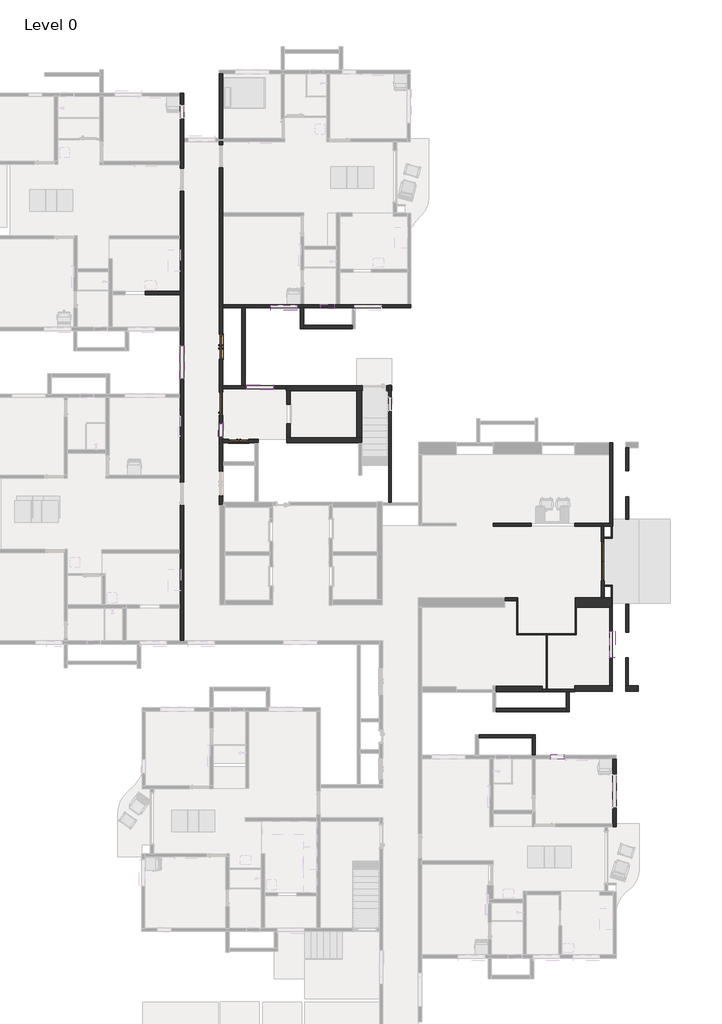
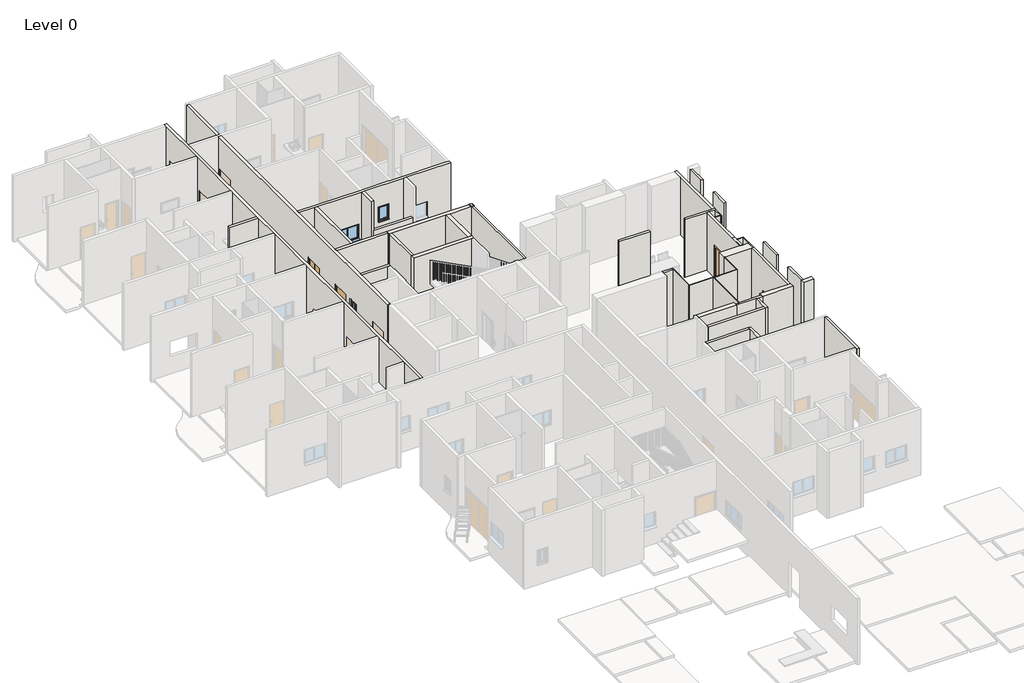
# One storey, part 6 of 14: 43 walls, 7 windows, 4 doors.
# Revit data of these elements (continued)
# Type "Windows_Tpl_Variable_Casement : 2'" (continued)
#   Analytic Construction = "1/8 in Pilkington single glazing"
#   Wrap Layers (Int) from Ext = 177.5 mm
#   Wrap Layers (Ext) from Ext = 102.5 mm
#   Window Board Projection = 25 mm
#   Window Board Extension = 25 mm
#   Visual Light Transmittance = 0.9
#   Solar Heat Gain Coefficient = 0.78
#   Rough Width = 609.6 mm
#   Rough Height = 910 mm
#   Height = 910 mm
#   Width = 609.6 mm
#   Heat Transfer Coefficient (U) = 3.6886 W/(m²·K)
#   Glazing Thickness = 24 mm
#   FrameOffset - External = 50 mm
#   Frame Depth = 65 mm
#   Default Head Height = 2110 mm
#   Cill Depth = 87.5 mm
#   Cavity Closer Width = 50 mm
#   Cavity Closer Offset from Ext = 102.5 mm
#   Cavity Closer Depth = 85 mm
#   Casement Width = 450 mm
#   Vis - Cavity Closers = yes
#   Define Thermal Properties by = 1
#   Material Trim = Window Frame
#   Material Glass = Glass
#   Material Frame = Window Frame
#   Wall Closure = (empty or 0)
# Type "Windows_Tpl_Variable_Casement : 4'"
#   Type Mark = "81"
#   Operation = "TriplePanelVertical"
#   Construction Type Id = "GSP4R"
#   Manufacturer = "Revit"
#   Keynote = "L10"
#   Analytic Construction = "1/8 in Pilkington single glazing"
#   Wrap Layers (Int) from Ext = 177.5 mm
#   Wrap Layers (Ext) from Ext = 102.5 mm
#   Window Board Projection = 25 mm
#   Window Board Extension = 25 mm
#   Visual Light Transmittance = 0.9
#   Solar Heat Gain Coefficient = 0.78
#   Rough Width = 1219.2 mm
#   Rough Height = 910 mm
#   Height = 910 mm
#   Width = 1219.2 mm
#   Heat Transfer Coefficient (U) = 3.6886 W/(m²·K)
#   Glazing Thickness = 24 mm
#   FrameOffset - External = 50 mm
#   Frame Depth = 65 mm
#   Default Head Height = 2110 mm
#   Cill Depth = 87.5 mm
#   Cavity Closer Width = 50 mm
#   Cavity Closer Offset from Ext = 102.5 mm
#   Cavity Closer Depth = 85 mm
#   Casement Width = 450 mm
#   Vis - Cavity Closers = yes
#   Define Thermal Properties by = 1
#   Material Trim = Window Frame
#   Material Glass = Glass
#   Material Frame = Window Frame
#   Wall Closure = (empty or 0)
# Type "Windows_Tpl_Variable_Casement : 5'"
#   Type Mark = "83"
#   Operation = "TriplePanelVertical"
#   Construction Type Id = "GSP4R"
#   Manufacturer = "Revit"
#   Keynote = "L10"
#   Analytic Construction = "1/8 in Pilkington single glazing"
#   Wrap Layers (Int) from Ext = 177.5 mm
#   Wrap Layers (Ext) from Ext = 102.5 mm
#   Window Board Projection = 25 mm
#   Window Board Extension = 25 mm
#   Visual Light Transmittance = 0.9
#   Solar Heat Gain Coefficient = 0.78
#   Rough Width = 1524 mm
#   Rough Height = 910 mm
#   Height = 910 mm
#   Width = 1524 mm
#   Heat Transfer Coefficient (U) = 3.6886 W/(m²·K)
#   Glazing Thickness = 24 mm
#   FrameOffset - External = 50 mm
#   Frame Depth = 65 mm
#   Default Head Height = 2110 mm
#   Cill Depth = 87.5 mm
#   Cavity Closer Width = 50 mm
#   Cavity Closer Offset from Ext = 102.5 mm
#   Cavity Closer Depth = 85 mm
#   Casement Width = 450 mm
#   Vis - Cavity Closers = yes
#   Define Thermal Properties by = 1
#   Material Trim = Window Frame
#   Material Glass = Glass
#   Material Frame = Window Frame
#   Wall Closure = (empty or 0)
# Element 1 (IfcDoor, "Doors_ExtDbl_Flush : 1810x2110mm")
#   Phase Created = New Construction
#   Materials on its faces: "Door - Handle", "Door - Frame/Mullion", "Door - Panel"
# Element 2 (IfcDoor, "Doors_ExtDbl_Flush : 3'")
#   Phase Created = New Construction
#   Materials on its faces: "Door - Handle", "Door - Frame/Mullion", "Door - Panel"
# Element 3 (IfcDoor, "Doors_ExtDbl_Flush : 3.75'")
#   Phase Created = New Construction
#   Materials on its faces: "Door - Handle", "Door - Frame/Mullion", "Door - Panel"
# Element 4 (IfcDoor, "Doors_ExtSgl_Flush : D1")
#   Phase Created = New Construction
#   Materials on its faces: "Door - Handle", "Door - Frame/Mullion", "Door - Panel"
# Elements 5, 6, 7, 8, 9, 10, 11, 12, 13, 14, 15, 17, 18 (IfcWall, "W1")
#   Top Offset = 0 mm
#   Base Offset = 0 mm
#   wall height = 4000 mm
#   Phase Created = New Construction
#   Base Constraint = Level 0
#   Top Constraint = Level 1
#   Materials on its faces: "Brick, Common"
# Element 16 (IfcWall, "W1")
#   Top Offset = -1828.8 mm
#   Base Offset = 0 mm
#   wall height = 2171.2 mm
#   Phase Created = New Construction
#   Base Constraint = Level 0
#   Top Constraint = Level 1
#   Materials on its faces: "Brick, Common"
# Elements 19, 20, 21, 22, 23, 24, 25, 26 (IfcWall, "W2")
#   Top Offset = 0 mm
#   Base Offset = 0 mm
#   wall height = 4000 mm
#   Phase Created = New Construction
#   Base Constraint = Level 0
#   Top Constraint = Level 1
#   Materials on its faces: "Brick, Common"
# Elements 27, 28, 29 (IfcWall, "W3")
#   Top Offset = 0 mm
#   Base Offset = 0 mm
#   wall height = 4000 mm
#   Phase Created = New Construction
#   Base Constraint = Level 0
#   Top Constraint = Level 1
#   Materials on its faces: "Brick, Common"
# Elements 30, 31, 32 (IfcWall, "W5")
#   Top Offset = 0 mm
#   Base Offset = 0 mm
#   wall height = 4000 mm
#   Phase Created = New Construction
#   Base Constraint = Level 0
#   Top Constraint = Level 1
#   Materials on its faces: "Brick, Common"
# Elements 33, 34, 35, 36, 37, 38, 39, 40, 41, 42, 43, 44, 45, 46 (IfcWall, "W6")
#   Top Offset = 0 mm
#   Base Offset = 0 mm
#   wall height = 4000 mm
#   Phase Created = New Construction
#   Base Constraint = Level 0
#   Top Constraint = Level 1
#   Materials on its faces: "Brick, Common"
# Element 47 (IfcWall, "W8")
#   Top Offset = 0 mm
#   Base Offset = 0 mm
#   wall height = 4000 mm
#   Phase Created = New Construction
#   Base Constraint = Level 0
#   Top Constraint = Level 1
#   Materials on its faces: "Brick, Common"
# Element 48 (IfcWindow, "Windows_Concept_Plain_Dbl : 4'")
#   Mark = "36"
#   Phase Created = New Construction
#   Materials on its faces: "Window Frame", "Glass"
# Element 49 (IfcWindow, "Windows_Concept_Plain_Dbl : 4'")
#   Mark = "32"
#   Phase Created = New Construction
#   Materials on its faces: "Window Frame", "Glass"
# Element 50 (IfcWindow, "Windows_Sgl_Plain : 2'")
#   Mark = "40"
#   Phase Created = New Construction
#   Materials on its faces: "Window Frame", "Glass"
# Element 51 (IfcWindow, "Windows_Tpl_Variable_Casement : 2'")
#   Mark = "31"
#   Phase Created = New Construction
#   Materials on its faces: "Window Frame", "Glass"
# Element 52 (IfcWindow, "Windows_Tpl_Variable_Casement : 2'")
#   Mark = "34"
#   Phase Created = New Construction
#   Materials on its faces: "Window Frame", "Glass"
# Element 53 (IfcWindow, "Windows_Tpl_Variable_Casement : 4'")
#   Mark = "73"
#   Phase Created = New Construction
#   Materials on its faces: "Window Frame", "Glass"
# Element 54 (IfcWindow, "Windows_Tpl_Variable_Casement : 5'")
#   Mark = "71"
#   Phase Created = New Construction
#   Materials on its faces: "Window Frame", "Glass"
# Materials
#   "Door - Panel": class "Wood", colour RGB 210 159 95, transparency 0, Keynote = "L20", Cost = 0
#   "Door - Frame/Mullion": class "Wood", colour RGB 212 179 113, transparency 0, Keynote = "L20", Cost = 0
#   "Door - Handle": colour RGB 0 0 0, transparency 0, Keynote = "P21", Cost = 0
#   "Brick, Common": class "Masonry", colour RGB 170 100 105, transparency 0, Description = "Common brick", Cost = 0
#   "Window Frame": colour RGB 249 249 249, transparency 0, Keynote = "L10", Cost = 0
#   "Glass": class "Glass", colour RGB 0 128 192, transparency 0.9, Description = "Soda Lime Glass", Cost = 0
